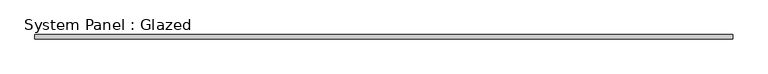
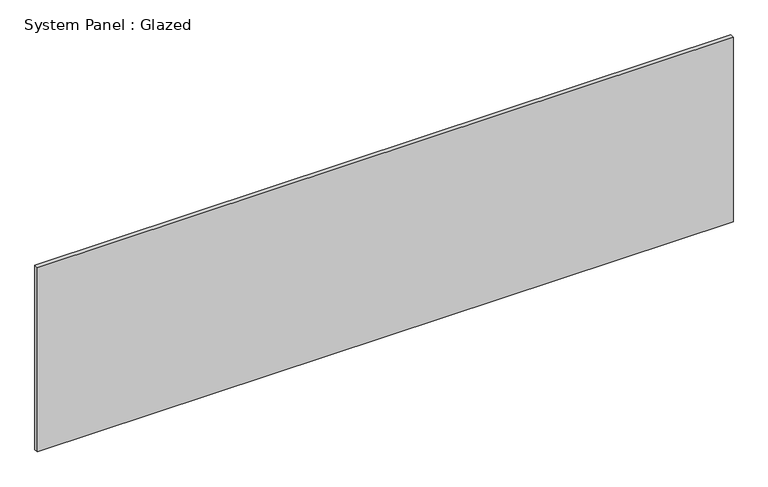
"""IFC4 building model written with IfcOpenShell, lengths in millimetres: plate geometry, System Panel : Glazed."""

from ifc_helpers import new_model, si_unit, origin, origin_with_axes, place, context, project, spatial, polyline, outline, extrude, source, transform, mapped, element, save


def system_panel_glazed_3acda581(model_context):
    return source(origin(), model_context, "Body", "SweptSolid", [
        extrude(outline(polyline([(2089.15, 19.05), (-2089.15, 19.05), (-2089.15, 44.45), (2089.15, 44.45), (2089.15, 19.05)])), origin_with_axes(), (0.0, 0.0, 1.0), 1169.7619602),
    ])


if __name__ == "__main__":
    model = new_model("IFC4")
    model_context = context("Model", 3, world=origin())
    ifc_project = project(units=[si_unit("LENGTHUNIT", "METRE", prefix="MILLI")], contexts=[model_context])
    site = spatial("IfcSite", under=ifc_project)
    building = spatial("IfcBuilding", under=site)
    placement = place(None, origin())
    system_panel_glazed_shape = system_panel_glazed_3acda581(model_context)
    element("IfcPlate", 1, ObjectType="System Panel : Glazed", at=placement, inside=building, context=model_context, shape_type="MappedRepresentation", body=[
        mapped(system_panel_glazed_shape, transform((0.0, 0.0, 0.0), x_axis=(1.0, 0.0, 0.0), y_axis=(0.0, 1.0, 0.0), z_axis=(0.0, 0.0, 1.0))),
    ])
    save(model, "model.ifc")

# Revit data of these elements
# Type "System Panel : Glazed"
#   Construction Type Id = "GSP4R"
#   Analytic Construction = "1/8 in Pilkington single glazing"
#   Visual Light Transmittance = 0.9
#   Solar Heat Gain Coefficient = 0.86
#   Heat Transfer Coefficient (U) = 1.18115 BTU/(h·ft²·°F)
#   Define Thermal Properties by = 1
# Element 1 (IfcPlate, "System Panel : Glazed")
#   Materials on its faces: "Glass"
# Materials
#   "Glass": class "Glass", colour RGB 0 128 192, transparency 0.75, Description = "Soda Lime Glass", Cost = 0
